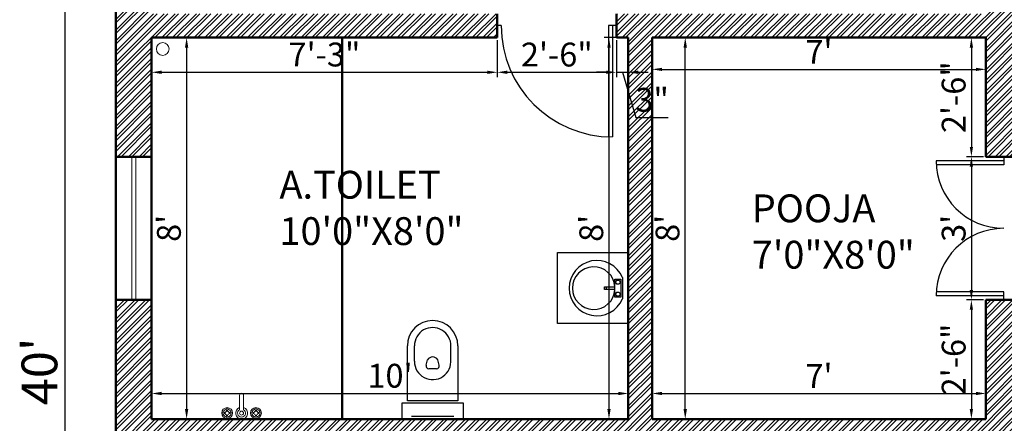
# Model space of a CAD drawing. Units: inches. Extents: x 3590 to 5167, y 65 to 1917.
# Tile 3 of 100: x 3621 to 3869, y 336 to 438. Entities that reach past the tile are written whole.
import ezdxf

# ---------------------------------------------------------------- set-up
doc = ezdxf.new("R2010")
doc.units = ezdxf.units.IN
for name, color, linetype, lineweight in [('A-ANNO-DIMS', 2, 'Continuous', 18), ('A-AREA-IDEN', 7, 'Continuous', 18), ('A-DOOR', 3, 'Continuous', 25), ('A-FLOR-FIXT', 8, 'Continuous', 18), ('A-GLAZ', 4, 'Continuous', 18), ('A-WALL', 7, 'Continuous', 50), ('A-WALL-PATT', 251, 'Continuous', 13)]:
    doc.layers.add(name, color=color, linetype=linetype, lineweight=lineweight)
doc.layers.add('SANTEH', color=7, linetype='Continuous')
doc.styles.get("Standard").update_dxf_attribs({"font": 'arial.ttf'})
doc.dimstyles.new('ISO-25', dxfattribs={"dimtxt": 9, "dimasz": 2.5, "dimexe": 1.25, "dimexo": 0.625, "dimtad": 1, "dimdec": 1, "dimlunit": 3, "dimtxsty": 'Standard', "dimcen": 2.5, "dimadec": 0, "dimazin": 0, "dimtfac": 1, "dimtdec": 1, "dimtmove": 0, "dimatfit": 3, "dimfxl": 1, "dimarcsym": 0})

# ---------------------------------------------------------------- blocks, each defined once
blk = doc.blocks.new('*D248')
at = {"layer": 'A-ANNO-DIMS', "color": 0, "lineweight": -2, "transparency": 16777216}
for p, q in [((3644.89, 589.06), (3631.39, 589.06)), ((3632.64, 586.56), (3632.64, 111.56)), ((3644.89, 109.06), (3631.39, 109.06))]:
    blk.add_line(p, q, dxfattribs=at)
at = {"layer": 'A-ANNO-DIMS', "color": 0, "transparency": 16777216}
for points in [[(3632.22, 586.56), (3633.06, 586.56), (3632.64, 589.06)], [(3632.22, 111.56), (3633.06, 111.56), (3632.64, 109.06)]]:
    blk.add_solid(points, dxfattribs=at)
at = {"layer": 'Defpoints', "color": 0, "transparency": 16777216}
for p in [(3645.51, 589.06), (3632.64, 109.06), (3645.51, 109.06)]:
    blk.add_point(p, dxfattribs=at)
at = {"layer": 'A-ANNO-DIMS', "color": 0, "transparency": 16777216, "insert": (3627.42, 349.06), "char_height": 9, "attachment_point": 5, "rotation": 90}
blk.add_mtext("40'", dxfattribs=at)
blk = doc.blocks.new('D2')
for p, q in [((1, 0), (1, 28)), ((2, 0), (2, 27.98)), ((0, 0), (2, 0)), ((29, 0), (30, 0))]:
    blk.add_line(p, q)
at = {"ltscale": 0.5}
blk.add_arc((1, 0), 28, 0, 90, dxfattribs=at)
blk = doc.blocks.new('D3')
for p, q in [((1, 0), (1, 17)), ((2, 0), (2, 16.97)), ((34, 0), (34, 16.97)), ((35, 0), (35, 17)), ((0, 0), (2, 0)), ((36, 0), (34, 0))]:
    blk.add_line(p, q)
at = {"ltscale": 0.5}
for centre, start, end in [((1, 0), 0, 90), ((35, 0), 90, 180)]:
    blk.add_arc(centre, 17, start, end, dxfattribs=at)
blk = doc.blocks.new('*D208')
at = {"layer": 'A-ANNO-DIMS', "color": 0, "lineweight": -2, "transparency": 16777216}
for p, q in [((3654.51, 432.43), (3654.51, 423.08)), ((3741.51, 432.43), (3741.51, 423.08)), ((3657.01, 424.33), (3739.01, 424.33))]:
    blk.add_line(p, q, dxfattribs=at)
at = {"layer": 'A-ANNO-DIMS', "color": 0, "transparency": 16777216}
for points in [[(3657.01, 424.74), (3657.01, 423.91), (3654.51, 424.33)], [(3739.01, 424.74), (3739.01, 423.91), (3741.51, 424.33)]]:
    blk.add_solid(points, dxfattribs=at)
at = {"layer": 'Defpoints', "color": 0, "transparency": 16777216}
for p in [(3654.51, 433.06), (3741.51, 433.06), (3741.51, 424.33)]:
    blk.add_point(p, dxfattribs=at)
at = {"layer": 'A-ANNO-DIMS', "color": 0, "transparency": 16777216, "insert": (3698.01, 428.02), "char_height": 6, "attachment_point": 5}
blk.add_mtext('7\'-3"', dxfattribs=at)
blk = doc.blocks.new('*D209')
at = {"layer": 'A-ANNO-DIMS', "color": 0, "lineweight": -2, "transparency": 16777216}
for p, q in [((3741.51, 432.43), (3741.51, 423.08)), ((3771.51, 432.43), (3771.51, 423.08)), ((3744.01, 424.33), (3769.01, 424.33))]:
    blk.add_line(p, q, dxfattribs=at)
at = {"layer": 'A-ANNO-DIMS', "color": 0, "transparency": 16777216}
for points in [[(3744.01, 424.74), (3744.01, 423.91), (3741.51, 424.33)], [(3769.01, 424.74), (3769.01, 423.91), (3771.51, 424.33)]]:
    blk.add_solid(points, dxfattribs=at)
at = {"layer": 'Defpoints', "color": 0, "transparency": 16777216}
for p in [(3741.51, 433.06), (3771.51, 433.06), (3771.51, 424.33)]:
    blk.add_point(p, dxfattribs=at)
at = {"layer": 'A-ANNO-DIMS', "color": 0, "transparency": 16777216, "insert": (3756.51, 428.01), "char_height": 6, "attachment_point": 5}
blk.add_mtext('2\'-6"', dxfattribs=at)
blk = doc.blocks.new('*D210')
at = {"layer": 'A-ANNO-DIMS', "color": 0, "lineweight": -2, "transparency": 16777216}
for p, q in [((3771.51, 432.43), (3771.51, 423.08)), ((3774.51, 432.43), (3774.51, 423.08)), ((3769.01, 424.33), (3766.51, 424.33)), ((3771.51, 424.33), (3774.51, 424.33)), ((3771.51, 424.33), (3774.51, 424.33)), ((3773.01, 424.33), (3776.43, 412.94)), ((3777.01, 424.33), (3779.51, 424.33)), ((3776.43, 412.94), (3784.57, 412.94))]:
    blk.add_line(p, q, dxfattribs=at)
at = {"layer": 'A-ANNO-DIMS', "color": 0, "transparency": 16777216}
for points in [[(3769.01, 424.74), (3769.01, 423.91), (3771.51, 424.33)], [(3777.01, 424.74), (3777.01, 423.91), (3774.51, 424.33)]]:
    blk.add_solid(points, dxfattribs=at)
at = {"layer": 'Defpoints', "color": 0, "transparency": 16777216}
for p in [(3771.51, 433.06), (3774.51, 433.06), (3774.51, 424.33)]:
    blk.add_point(p, dxfattribs=at)
at = {"layer": 'A-ANNO-DIMS', "color": 0, "transparency": 16777216, "insert": (3780.5, 416.63), "char_height": 6, "attachment_point": 5}
blk.add_mtext('3"', dxfattribs=at)
blk = doc.blocks.new('*D211')
at = {"layer": 'A-ANNO-DIMS', "color": 0, "lineweight": -2, "transparency": 16777216}
for p, q in [((3655.14, 433.06), (3664.56, 433.06)), ((3663.31, 430.56), (3663.31, 339.56)), ((3655.14, 337.06), (3664.56, 337.06))]:
    blk.add_line(p, q, dxfattribs=at)
at = {"layer": 'A-ANNO-DIMS', "color": 0, "transparency": 16777216}
for points in [[(3662.89, 430.56), (3663.72, 430.56), (3663.31, 433.06)], [(3662.89, 339.56), (3663.72, 339.56), (3663.31, 337.06)]]:
    blk.add_solid(points, dxfattribs=at)
at = {"layer": 'Defpoints', "color": 0, "transparency": 16777216}
for p in [(3654.51, 433.06), (3654.51, 337.06), (3663.31, 337.06)]:
    blk.add_point(p, dxfattribs=at)
at = {"layer": 'A-ANNO-DIMS', "color": 0, "transparency": 16777216, "insert": (3659.62, 385.06), "char_height": 6, "attachment_point": 5, "rotation": 90}
blk.add_mtext("8'", dxfattribs=at)
blk = doc.blocks.new('*D212')
at = {"layer": 'A-ANNO-DIMS', "color": 0, "lineweight": -2, "transparency": 16777216}
for p, q in [((3654.51, 337.68), (3654.51, 344.75)), ((3774.51, 337.68), (3774.51, 344.75)), ((3657.01, 343.5), (3772.01, 343.5))]:
    blk.add_line(p, q, dxfattribs=at)
at = {"layer": 'A-ANNO-DIMS', "color": 0, "transparency": 16777216}
for points in [[(3657.01, 343.92), (3657.01, 343.08), (3654.51, 343.5)], [(3772.01, 343.92), (3772.01, 343.08), (3774.51, 343.5)]]:
    blk.add_solid(points, dxfattribs=at)
at = {"layer": 'Defpoints', "color": 0, "transparency": 16777216}
for p in [(3774.51, 343.5), (3654.51, 337.06), (3774.51, 337.06)]:
    blk.add_point(p, dxfattribs=at)
at = {"layer": 'A-ANNO-DIMS', "color": 0, "transparency": 16777216, "insert": (3714.51, 347.19), "char_height": 6, "attachment_point": 5}
blk.add_mtext("10'", dxfattribs=at)
blk = doc.blocks.new('*D203')
at = {"layer": 'A-ANNO-DIMS', "color": 0, "lineweight": -2, "transparency": 16777216}
for p, q in [((3780.51, 337.68), (3780.51, 344.75)), ((3864.51, 337.68), (3864.51, 344.75)), ((3783.01, 343.5), (3862.01, 343.5))]:
    blk.add_line(p, q, dxfattribs=at)
at = {"layer": 'A-ANNO-DIMS', "color": 0, "transparency": 16777216}
for points in [[(3783.01, 343.92), (3783.01, 343.08), (3780.51, 343.5)], [(3862.01, 343.92), (3862.01, 343.08), (3864.51, 343.5)]]:
    blk.add_solid(points, dxfattribs=at)
at = {"layer": 'Defpoints', "color": 0, "transparency": 16777216}
for p in [(3864.51, 343.5), (3780.51, 337.06), (3864.51, 337.06)]:
    blk.add_point(p, dxfattribs=at)
at = {"layer": 'A-ANNO-DIMS', "color": 0, "transparency": 16777216, "insert": (3822.51, 347.13), "char_height": 6, "attachment_point": 5}
blk.add_mtext("7'", dxfattribs=at)
blk = doc.blocks.new('*D204')
at = {"layer": 'A-ANNO-DIMS', "color": 0, "lineweight": -2, "transparency": 16777216}
for p, q in [((3781.14, 433.06), (3790.09, 433.06)), ((3788.84, 339.56), (3788.84, 430.56)), ((3781.14, 337.06), (3790.09, 337.06))]:
    blk.add_line(p, q, dxfattribs=at)
at = {"layer": 'A-ANNO-DIMS', "color": 0, "transparency": 16777216}
for points in [[(3788.42, 430.56), (3789.26, 430.56), (3788.84, 433.06)], [(3788.42, 339.56), (3789.26, 339.56), (3788.84, 337.06)]]:
    blk.add_solid(points, dxfattribs=at)
at = {"layer": 'Defpoints', "color": 0, "transparency": 16777216}
for p in [(3780.51, 433.06), (3788.84, 433.06), (3780.51, 337.06)]:
    blk.add_point(p, dxfattribs=at)
at = {"layer": 'A-ANNO-DIMS', "color": 0, "transparency": 16777216, "insert": (3785.15, 385.06), "char_height": 6, "attachment_point": 5, "rotation": 90}
blk.add_mtext("8'", dxfattribs=at)
blk = doc.blocks.new('*D205')
at = {"layer": 'A-ANNO-DIMS', "color": 0, "lineweight": -2, "transparency": 16777216}
for p, q in [((3773.89, 433.06), (3768.39, 433.06)), ((3769.64, 430.56), (3769.64, 339.56)), ((3773.89, 337.06), (3768.39, 337.06))]:
    blk.add_line(p, q, dxfattribs=at)
at = {"layer": 'A-ANNO-DIMS', "color": 0, "transparency": 16777216}
for points in [[(3769.23, 430.56), (3770.06, 430.56), (3769.64, 433.06)], [(3769.23, 339.56), (3770.06, 339.56), (3769.64, 337.06)]]:
    blk.add_solid(points, dxfattribs=at)
at = {"layer": 'Defpoints', "color": 0, "transparency": 16777216}
for p in [(3774.51, 433.06), (3769.64, 337.06), (3774.51, 337.06)]:
    blk.add_point(p, dxfattribs=at)
at = {"layer": 'A-ANNO-DIMS', "color": 0, "transparency": 16777216, "insert": (3765.96, 385.06), "char_height": 6, "attachment_point": 5, "rotation": 90}
blk.add_mtext("8'", dxfattribs=at)
blk = doc.blocks.new('*D206')
at = {"layer": 'A-ANNO-DIMS', "color": 0, "lineweight": -2, "transparency": 16777216}
for p, q in [((3780.51, 432.43), (3780.51, 423.81)), ((3864.51, 432.43), (3864.51, 423.81)), ((3783.01, 425.06), (3862.01, 425.06))]:
    blk.add_line(p, q, dxfattribs=at)
at = {"layer": 'A-ANNO-DIMS', "color": 0, "transparency": 16777216}
for points in [[(3783.01, 425.47), (3783.01, 424.64), (3780.51, 425.06)], [(3862.01, 425.47), (3862.01, 424.64), (3864.51, 425.06)]]:
    blk.add_solid(points, dxfattribs=at)
at = {"layer": 'Defpoints', "color": 0, "transparency": 16777216}
for p in [(3780.51, 433.06), (3864.51, 433.06), (3864.51, 425.06)]:
    blk.add_point(p, dxfattribs=at)
at = {"layer": 'A-ANNO-DIMS', "color": 0, "transparency": 16777216, "insert": (3822.51, 428.68), "char_height": 6, "attachment_point": 5}
blk.add_mtext("7'", dxfattribs=at)
blk = doc.blocks.new('*D207')
at = {"layer": 'A-ANNO-DIMS', "color": 0, "lineweight": -2, "transparency": 16777216}
for p, q in [((3863.89, 433.06), (3859.63, 433.06)), ((3860.88, 430.56), (3860.88, 405.56)), ((3863.89, 403.06), (3859.63, 403.06))]:
    blk.add_line(p, q, dxfattribs=at)
at = {"layer": 'A-ANNO-DIMS', "color": 0, "transparency": 16777216}
for points in [[(3860.46, 430.56), (3861.29, 430.56), (3860.88, 433.06)], [(3860.46, 405.56), (3861.29, 405.56), (3860.88, 403.06)]]:
    blk.add_solid(points, dxfattribs=at)
at = {"layer": 'Defpoints', "color": 0, "transparency": 16777216}
for p in [(3864.51, 433.06), (3860.88, 403.06), (3864.51, 403.06)]:
    blk.add_point(p, dxfattribs=at)
at = {"layer": 'A-ANNO-DIMS', "color": 0, "transparency": 16777216, "insert": (3857.19, 418.06), "char_height": 6, "attachment_point": 5, "rotation": 90}
blk.add_mtext('2\'-6"', dxfattribs=at)
blk = doc.blocks.new('*D238')
at = {"layer": 'A-ANNO-DIMS', "color": 0, "lineweight": -2, "transparency": 16777216}
for p, q in [((3863.89, 403.06), (3859.63, 403.06)), ((3860.88, 400.56), (3860.88, 369.56)), ((3863.89, 367.06), (3859.63, 367.06))]:
    blk.add_line(p, q, dxfattribs=at)
at = {"layer": 'A-ANNO-DIMS', "color": 0, "transparency": 16777216}
for points in [[(3860.46, 400.56), (3861.29, 400.56), (3860.88, 403.06)], [(3860.46, 369.56), (3861.29, 369.56), (3860.88, 367.06)]]:
    blk.add_solid(points, dxfattribs=at)
at = {"layer": 'Defpoints', "color": 0, "transparency": 16777216}
for p in [(3864.51, 403.06), (3860.88, 367.06), (3864.51, 367.06)]:
    blk.add_point(p, dxfattribs=at)
at = {"layer": 'A-ANNO-DIMS', "color": 0, "transparency": 16777216, "insert": (3857.19, 385.06), "char_height": 6, "attachment_point": 5, "rotation": 90}
blk.add_mtext("3'", dxfattribs=at)
blk = doc.blocks.new('*D239')
at = {"layer": 'A-ANNO-DIMS', "color": 0, "lineweight": -2, "transparency": 16777216}
for p, q in [((3863.89, 367.06), (3859.63, 367.06)), ((3860.88, 364.56), (3860.88, 339.56)), ((3863.89, 337.06), (3859.63, 337.06))]:
    blk.add_line(p, q, dxfattribs=at)
at = {"layer": 'A-ANNO-DIMS', "color": 0, "transparency": 16777216}
for points in [[(3860.46, 364.56), (3861.29, 364.56), (3860.88, 367.06)], [(3860.46, 339.56), (3861.29, 339.56), (3860.88, 337.06)]]:
    blk.add_solid(points, dxfattribs=at)
at = {"layer": 'Defpoints', "color": 0, "transparency": 16777216}
for p in [(3864.51, 367.06), (3860.88, 337.06), (3864.51, 337.06)]:
    blk.add_point(p, dxfattribs=at)
at = {"layer": 'A-ANNO-DIMS', "color": 0, "transparency": 16777216, "insert": (3857.19, 352.06), "char_height": 6, "attachment_point": 5, "rotation": 90}
blk.add_mtext('2\'-6"', dxfattribs=at)
blk = doc.blocks.new('Faucet - Bathroom top')
for p, q in [((-4.107, 0.125), (-4.375, 0.125)), ((-3.75, 0.4788), (-3.75, 0.75)), ((-3.5, 0.482), (-3.5, 0.75)), ((-3.1461, 0.125), (-2.875, 0.125)), ((3.143, 0.125), (2.875, 0.125)), ((3.5, 0.4788), (3.5, 0.75)), ((3.75, 0.482), (3.75, 0.75)), ((4.1039, 0.125), (4.375, 0.125)), ((-4.1039, -0.125), (-4.375, -0.125)), ((-3.75, -0.4821), (-3.75, -0.75)), ((-3.5, -0.4789), (-3.5, -0.75)), ((-3.143, -0.125), (-2.875, -0.125)), ((-0.5, -0.8639), (-0.5, -4.5)), ((0.5, -4.5), (0.5, -0.8631)), ((3.1461, -0.125), (2.875, -0.125)), ((3.5, -0.4821), (3.5, -0.75)), ((3.75, -0.4789), (3.75, -0.75)), ((4.107, -0.125), (4.375, -0.125))]:
    blk.add_line(p, q)
for centre, radius in [((-3.625, 0), 1.375), ((-4.625, 0), 0.2795), ((-3.625, 0), 0.5), ((-3.625, 1), 0.2795), ((-2.625, 0), 0.2795), ((0, 0), 0.5), ((3.625, 0), 1.375), ((2.625, 0), 0.2795), ((3.625, 0), 0.5), ((3.625, 1), 0.2795), ((4.625, 0), 0.2795), ((-3.625, -1), 0.2795), ((3.625, -1), 0.2795)]:
    blk.add_circle(centre, radius)
for centre, radius, start, end in [((-3.625, 0), 1, 105.2407, 164.2093), ((-3.625, 0), 1, 16.44125, 74.07887), ((0, 0), 1.5, 289.6514, 250.3603), ((0, 0), 1, 300.3431, 239.7554), ((3.625, 0), 1, 106.12, 164.0884), ((3.625, 0), 1, 16.23422, 73.90469), ((-3.625, 0), 1, 196.2342, 253.9047), ((-3.625, 0), 1, 286.12, 344.0884), ((3.625, 0), 1, 196.4413, 254.0789), ((3.625, 0), 1, 285.2407, 344.2093), ((0, -4.5), 0.5, 180, 0)]:
    blk.add_arc(centre, radius, start, end)
blk = doc.blocks.new('y3')
at = {"layer": 'SANTEH', "ltscale": 5}
for p, q in [((37.5, 130.7), (37.5, 520.7)), ((87.5, 410.7), (87.5, 520.7)), ((346.6, 426.1), (347.5, 520.7)), ((397.5, 520.7), (397.5, 130.7)), ((171.9, 384.5), (181.1, 421.3)), ((263.1, 384.5), (253.9, 421.3)), ((244.3, 357.8), (190.7, 357.8)), ((397.5, 130.7), (37.5, 130.7)), ((67.5, 20.7), (367.5, 20.7))]:
    blk.add_line(p, q, dxfattribs=at)
blk.add_lwpolyline([(0, 115), (435, 115), (435, 0), (0, 0), (0, 115)], dxfattribs=at)
for centre, radius, start, end in [((217.5, 520.7), 180, 0, 180), ((217.5, 520.7), 130, 359.15795, 180), ((217.5, 410.7), 130, 180, 5.98548), ((217.5, 399.9), 42.2, 30.52342, 149.47658), ((190.7, 377.8), 20, 160.50385, 270), ((244.3, 377.8), 20, 270, 19.49615)]:
    blk.add_arc(centre, radius, start, end, dxfattribs=at)
blk = doc.blocks.new('r11')
at = {"layer": 'SANTEH', "ltscale": 5}
for p, q in [((0, 0), (600, 0)), ((0, -600), (0, 0)), ((600, 0), (600, -600)), ((210.5, -50), (389.5, -50)), ((210.5, -50), (210.5, -50)), ((223.8, -63.2), (376.2, -63.2)), ((223.8, -113.2), (223.8, -63.2)), ((232.7, -78.7), (249.2, -69.1)), ((232.7, -97.7), (232.7, -78.7)), ((249.2, -69.1), (265.7, -78.7)), ((265.7, -78.7), (265.7, -97.7)), ((334.3, -78.7), (350.8, -69.1)), ((334.3, -97.7), (334.3, -78.7)), ((350.8, -69.1), (367.3, -78.7)), ((367.3, -78.7), (367.3, -97.7)), ((376.2, -63.2), (376.2, -113.2)), ((376.2, -113.2), (223.8, -113.2)), ((249.2, -107.2), (232.7, -97.7)), ((265.7, -97.7), (249.2, -107.2)), ((288, -201.6), (288, -113.2)), ((312, -113.2), (312, -201.6)), ((350.8, -107.2), (334.3, -97.7)), ((367.3, -97.7), (350.8, -107.2)), ((312, -184.3), (288, -184.3)), ((312, -201.6), (288, -201.6)), ((600, -600), (0, -600))]:
    blk.add_line(p, q, dxfattribs=at)
for centre, radius, start, end in [((300, -266.2), 234, 112.50001, 67.49999), ((300, -293), 180.2, 93.8183, 86.1817)]:
    blk.add_arc(centre, radius, start, end, dxfattribs=at)

msp = doc.modelspace()

# ---------------------------------------------------------------- hatches: boundary and pattern name
at = {"layer": 'A-WALL-PATT', "transparency": 33554687}
h = msp.add_hatch(dxfattribs=at)
h.set_pattern_fill('ANSI32', color=256, scale=0.2)
h.set_pattern_definition([(45, (0, -1216.9392), (-1.3470384, 1.3470384), []), (45, (0.898, -1216.9392), (-1.3470384, 1.3470384), [])])
h.paths.add_polyline_path([(3768.51, 589.06), (3645.51, 589.06), (3645.51, 568.06), (3654.51, 568.06), (3654.51, 580.06), (3671.16, 580.06), (3768.51, 580.06)])
h.paths.add_polyline_path([(3909.51, 589.06), (3816.51, 589.06), (3816.51, 580.06), (3864.51, 580.06), (3864.51, 574.06), (3873.51, 574.06), (3873.51, 580.06), (3909.51, 580.06)])
h.paths.add_polyline_path([(4053.51, 589.06), (3969.51, 589.06), (3969.51, 580.06), (4053.51, 580.06)])
h.paths.add_polyline_path([(4215.51, 589.06), (4113.51, 589.06), (4113.51, 580.06), (4206.51, 580.06), (4206.51, 574.06), (4215.51, 574.06)])
h.paths.add_polyline_path([(3654.51, 520.06), (3645.51, 520.06), (3645.51, 403.06), (3654.51, 403.06), (3654.51, 433.06), (3741.51, 433.06), (3741.51, 439.06), (3654.51, 439.06)], flags=17)
h.paths.add_polyline_path([(3873.51, 538.06), (3864.51, 538.06), (3864.51, 439.06), (3771.51, 439.06), (3771.51, 433.06), (3774.51, 433.06), (3774.51, 337.06), (3654.51, 337.06), (3654.51, 367.06), (3645.51, 367.06), (3645.51, 322.06), (3654.51, 322.06), (3654.51, 328.06), (3864.51, 328.06), (3864.51, 322.06), (3873.51, 322.06), (3873.51, 367.06), (3864.51, 367.06), (3864.51, 337.06), (3780.51, 337.06), (3780.51, 433.06), (3864.51, 433.06), (3864.51, 403.06), (3873.51, 403.06)])
h.paths.add_polyline_path([(3654.51, 274.06), (3645.51, 274.06), (3645.51, 109.06), (3810.51, 109.06), (3810.51, 118.06), (3809.96, 118.06), (3654.51, 118.06)])
h.paths.add_polyline_path([(3915.51, 118.06), (3873.51, 118.06), (3873.51, 135.93), (3873.51, 205.06), (3876.51, 205.06), (3876.51, 214.06), (3864.51, 214.06), (3864.51, 118.06), (3858.51, 118.06), (3858.51, 109.06), (3915.51, 109.06)])
h.paths.add_polyline_path([(4028.01, 118.06), (4002.51, 118.06), (4002.51, 286.06), (3981.51, 286.06), (3981.51, 277.06), (3993.51, 277.06), (3993.51, 214.06), (3921.51, 214.06), (3921.51, 277.06), (3933.51, 277.06), (3933.51, 286.06), (3864.51, 286.06), (3864.51, 277.06), (3912.51, 277.06), (3912.51, 214.06), (3906.51, 214.06), (3906.51, 205.06), (3993.51, 205.06), (3993.51, 118.06), (3951.51, 118.06), (3951.51, 109.06), (4028.01, 109.06)])
h.paths.add_polyline_path([(4203.51, 118.06), (4158.51, 118.06), (4158.51, 310.06), (4194.51, 310.06), (4194.51, 319.06), (4149.51, 319.06), (4149.51, 118.06), (4124.01, 118.06), (4124.01, 109.06), (4203.51, 109.06)])
h.paths.add_polyline_path([(4305.51, 349.06), (4296.51, 349.06), (4296.51, 319.06), (4278.64, 319.06), (4260.51, 319.06), (4260.51, 310.06), (4296.51, 310.06), (4296.51, 304.06), (4305.51, 304.06)])
h.paths.add_polyline_path([(4305.51, 256.06), (4296.51, 256.06), (4296.51, 118.06), (4251.51, 118.06), (4251.51, 109.06), (4305.51, 109.06)])
h.paths.add_polyline_path([(4305.51, 460.06), (4215.51, 460.06), (4215.51, 526.06), (4206.51, 526.06), (4206.51, 460.06), (4149.51, 460.06), (4149.51, 451.06), (4296.51, 451.06), (4296.51, 421.06), (4305.51, 421.06)])

# ---------------------------------------------------------------- linework, layer by layer
at = {"layer": 'A-FLOR-FIXT'}
msp.add_circle((3657.31, 430.19), 1.6, dxfattribs=at)
at = {"layer": 'A-GLAZ'}
for p, q in [((3649.51, 367.06), (3649.51, 403.06)), ((3650.51, 367.06), (3650.51, 403.06))]:
    msp.add_line(p, q, dxfattribs=at)
at = {"layer": 'A-WALL'}
for p, q in [((3741.51, 433.06), (3741.51, 439.06)), ((3771.51, 433.06), (3771.51, 439.06)), ((3654.51, 433.06), (3741.51, 433.06)), ((3654.51, 337.06), (3654.51, 433.06)), ((3702.51, 337.06), (3702.51, 433.06)), ((3771.51, 433.06), (3774.51, 433.06)), ((3774.51, 337.06), (3774.51, 433.06)), ((3780.51, 433.06), (3864.51, 433.06)), ((3780.51, 337.06), (3780.51, 433.06)), ((3864.51, 403.06), (3864.51, 433.06)), ((3654.51, 403.06), (3645.51, 403.06)), ((3864.51, 403.06), (3873.51, 403.06)), ((3654.51, 367.06), (3645.51, 367.06)), ((3864.51, 337.06), (3864.51, 367.06)), ((3864.51, 367.06), (3873.51, 367.06)), ((3774.51, 337.06), (3654.51, 337.06)), ((3864.51, 337.06), (3780.51, 337.06))]:
    msp.add_line(p, q, dxfattribs=at)
msp.add_lwpolyline([(4305.51, 460.06), (4305.51, 109.06), (3645.51, 109.06), (3645.51, 589.06), (4215.51, 589.06)], dxfattribs=at)

# ---------------------------------------------------------------- block references
at = {"layer": 'A-DOOR'}
for name, p, rotation in [('D2', (3771.51, 436.06), 180), ('D3', (3869.01, 367.06), 90)]:
    msp.add_blockref(name, p, dxfattribs=dict(at, rotation=rotation))
at = {"layer": 'A-FLOR-FIXT', "xscale": 0.0297800069284724, "yscale": 0.0297800069284724, "zscale": 0.0297800069284724, "rotation": 270}
msp.add_blockref('r11', (3774.51, 378.94), dxfattribs=at)
at = {"layer": 'A-FLOR-FIXT', "xscale": 0.0353848906415677, "yscale": 0.0353848906415677, "zscale": 0.0353848906415677}
msp.add_blockref('y3', (3717.55, 337.06), dxfattribs=at)
at = {"layer": 'A-FLOR-FIXT', "xscale": -1, "rotation": 180}
msp.add_blockref('Faucet - Bathroom top', (3677.14, 338.56), dxfattribs=at)

# ---------------------------------------------------------------- texts
at = {"layer": 'A-AREA-IDEN', "char_height": 7, "attachment_point": 1}
for s, insert in [('{\\fTimes New Roman|b0|i0|c0|p18;A.TOILET\\P10\'0"X8\'0"}', (3686.68, 399.53)), ('{\\fTimes New Roman|b0|i0|c0|p18;POOJA\\P7\'0"X8\'0"}', (3805.59, 393.59))]:
    msp.add_mtext_dynamic_manual_height_columns(s, width=67.3508, gutter_width=12.5, heights=[0], dxfattribs=dict(at, insert=insert))

# ---------------------------------------------------------------- dimensions: what is measured, and where the dimension line sits
at = {"layer": 'A-ANNO-DIMS'}
for base, p1, p2, override, picture, middle in [((3632.64, 109.06), (3645.51, 589.06), (3645.51, 109.06), {"dimclrd": 0, "dimclre": 0, "dimclrt": 0}, '*D248', (3627.42, 349.06)), ((3663.31, 337.06), (3654.51, 433.06), (3654.51, 337.06), {"dimtxt": 6, "dimclrd": 0, "dimclre": 0, "dimclrt": 0}, '*D211', (3659.62, 385.06)), ((3769.64, 337.06), (3774.51, 433.06), (3774.51, 337.06), {"dimtxt": 6, "dimclrd": 0, "dimclre": 0, "dimclrt": 0}, '*D205', (3765.96, 385.06)), ((3788.84, 433.06), (3780.51, 337.06), (3780.51, 433.06), {"dimtxt": 6, "dimclrd": 0, "dimclre": 0, "dimclrt": 0}, '*D204', (3785.15, 385.06)), ((3860.88, 403.06), (3864.51, 433.06), (3864.51, 403.06), {"dimtxt": 6, "dimclrd": 0, "dimclre": 0, "dimclrt": 0}, '*D207', (3857.19, 418.06)), ((3860.88, 367.06), (3864.51, 403.06), (3864.51, 367.06), {"dimtxt": 6, "dimclrd": 0, "dimclre": 0, "dimclrt": 0, "dimtmove": 1}, '*D238', (3857.19, 385.06)), ((3860.88, 337.06), (3864.51, 367.06), (3864.51, 337.06), {"dimtxt": 6, "dimclrd": 0, "dimclre": 0, "dimclrt": 0, "dimtmove": 1}, '*D239', (3857.19, 352.06))]:
    dim = msp.add_linear_dim(base=base, p1=p1, p2=p2, angle=90, dimstyle='ISO-25', override=override, dxfattribs=at)
    dim.commit()
    dim.dimension.update_dxf_attribs({"geometry": picture, "text_midpoint": middle})
for base, p1, p2, override, picture, middle in [((3741.51, 424.33), (3654.51, 433.06), (3741.51, 433.06), {"dimtxt": 6, "dimclrd": 0, "dimclre": 0, "dimclrt": 0}, '*D208', (3698.01, 428.02)), ((3771.51, 424.33), (3741.51, 433.06), (3771.51, 433.06), {"dimtxt": 6, "dimclrd": 0, "dimclre": 0, "dimclrt": 0, "dimtmove": 1}, '*D209', (3756.51, 428.01)), ((3774.51, 424.33), (3771.51, 433.06), (3774.51, 433.06), {"dimtxt": 6, "dimclrd": 0, "dimclre": 0, "dimclrt": 0, "dimtmove": 1}, '*D210', (3777.05, 416.63)), ((3864.51, 425.06), (3780.51, 433.06), (3864.51, 433.06), {"dimtxt": 6, "dimclrd": 0, "dimclre": 0, "dimclrt": 0}, '*D206', (3822.51, 428.68)), ((3774.51, 343.5), (3654.51, 337.06), (3774.51, 337.06), {"dimtxt": 6, "dimclrd": 0, "dimclre": 0, "dimclrt": 0}, '*D212', (3714.51, 347.19)), ((3864.51, 343.5), (3780.51, 337.06), (3864.51, 337.06), {"dimtxt": 6, "dimclrd": 0, "dimclre": 0, "dimclrt": 0}, '*D203', (3822.51, 347.13))]:
    dim = msp.add_linear_dim(base=base, p1=p1, p2=p2, dimstyle='ISO-25', override=override, dxfattribs=at)
    dim.commit()
    dim.dimension.update_dxf_attribs({"geometry": picture, "text_midpoint": middle})

doc.saveas('drawing.dxf')
